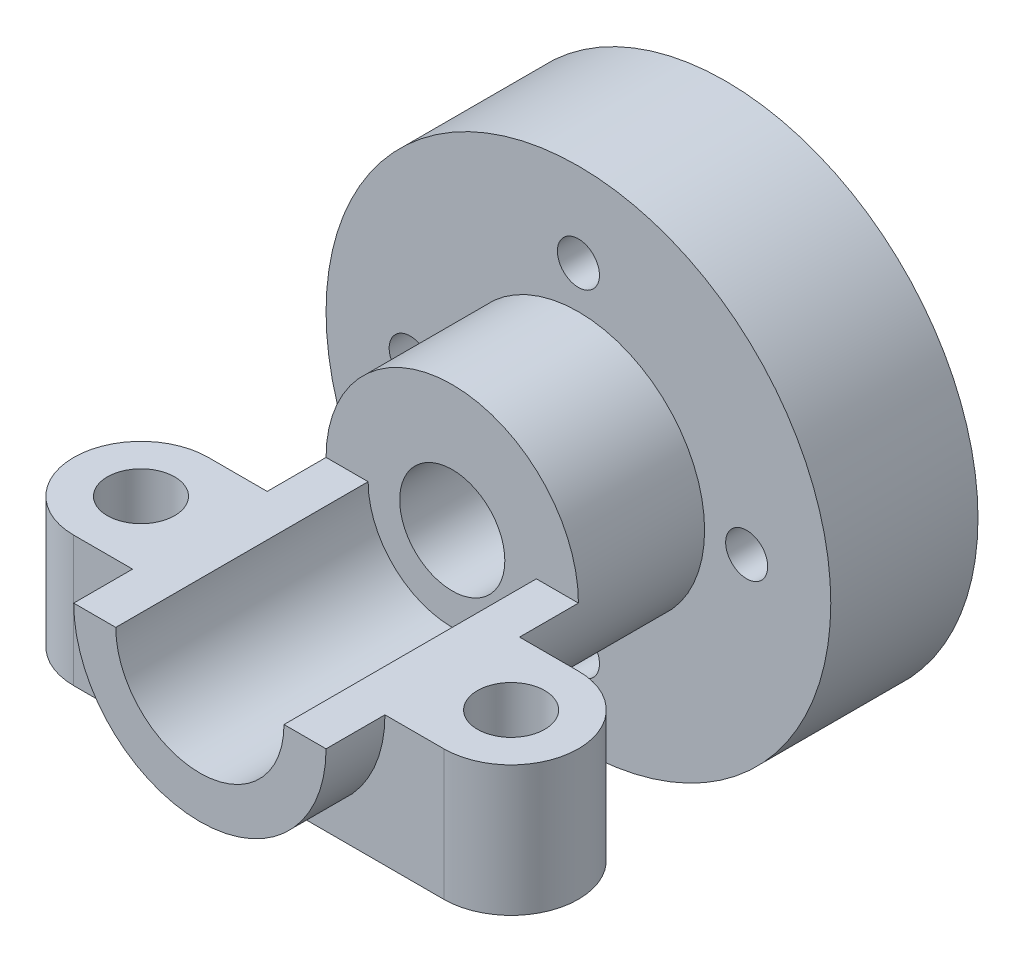
ISO-10303-21;
HEADER;
FILE_DESCRIPTION(('STEP AP214'),'2;1');
FILE_NAME('part.step','',(''),(''),'','','');
FILE_SCHEMA(('AUTOMOTIVE_DESIGN { 1 0 10303 214 1 1 1 1 }'));
ENDSEC;
DATA;
#1=APPLICATION_CONTEXT('core data for automotive mechanical design processes');
#2=APPLICATION_PROTOCOL_DEFINITION('international standard','automotive_design',2000,#1);
#3=PRODUCT_CONTEXT('',#1,'mechanical');
#4=PRODUCT('Part','Part','',(#3));
#5=PRODUCT_RELATED_PRODUCT_CATEGORY('part','',(#4));
#6=PRODUCT_DEFINITION_FORMATION('','',#4);
#7=PRODUCT_DEFINITION_CONTEXT('part definition',#1,'design');
#8=PRODUCT_DEFINITION('design','',#6,#7);
#9=PRODUCT_DEFINITION_SHAPE('','',#8);
#10=(LENGTH_UNIT() NAMED_UNIT(*) SI_UNIT(.MILLI.,.METRE.));
#11=(NAMED_UNIT(*) PLANE_ANGLE_UNIT() SI_UNIT($,.RADIAN.));
#12=(NAMED_UNIT(*) SI_UNIT($,.STERADIAN.) SOLID_ANGLE_UNIT());
#13=UNCERTAINTY_MEASURE_WITH_UNIT(LENGTH_MEASURE(1.E-05),#10,'distance_accuracy_value','');
#14=(GEOMETRIC_REPRESENTATION_CONTEXT(3) GLOBAL_UNCERTAINTY_ASSIGNED_CONTEXT((#13)) GLOBAL_UNIT_ASSIGNED_CONTEXT((#10,
#11,#12)) REPRESENTATION_CONTEXT('',''));
#15=CARTESIAN_POINT('',(0.,0.,0.));
#16=DIRECTION('',(0.,0.,1.));
#17=DIRECTION('',(1.,0.,0.));
#18=AXIS2_PLACEMENT_3D('',#15,#16,#17);
#19=CARTESIAN_POINT('',(-30.,0.,125.));
#20=DIRECTION('',(0.,-1.,0.));
#21=DIRECTION('',(0.,0.,-1.));
#22=AXIS2_PLACEMENT_3D('',#19,#20,#21);
#23=PLANE('',#22);
#24=CARTESIAN_POINT('',(44.,-1.39645239816133E-13,95.));
#25=DIRECTION('',(0.,-1.,0.));
#26=DIRECTION('',(0.,0.,-1.));
#27=AXIS2_PLACEMENT_3D('',#24,#25,#26);
#28=CIRCLE('',#27,8.);
#29=CARTESIAN_POINT('',(44.,-1.39645239816133E-13,87.));
#30=VERTEX_POINT('',#29);
#31=EDGE_CURVE('E51',#30,#30,#28,.T.);
#32=ORIENTED_EDGE('',*,*,#31,.T.);
#33=EDGE_LOOP('',(#32));
#34=FACE_BOUND('',#33,.T.);
#35=DIRECTION('',(0.,0.,1.));
#36=VECTOR('',#35,1.);
#37=CARTESIAN_POINT('',(20.,0.,65.));
#38=LINE('',#37,#36);
#39=CARTESIAN_POINT('',(20.,0.,65.));
#40=VERTEX_POINT('',#39);
#41=CARTESIAN_POINT('',(20.,0.,125.));
#42=VERTEX_POINT('',#41);
#43=EDGE_CURVE('E171',#40,#42,#38,.T.);
#44=ORIENTED_EDGE('',*,*,#43,.T.);
#45=DIRECTION('',(-1.,0.,0.));
#46=VECTOR('',#45,1.);
#47=CARTESIAN_POINT('',(12.5,0.,125.));
#48=LINE('',#47,#46);
#49=CARTESIAN_POINT('',(30.,0.,125.));
#50=VERTEX_POINT('',#49);
#51=EDGE_CURVE('E185',#50,#42,#48,.T.);
#52=ORIENTED_EDGE('',*,*,#51,.F.);
#53=DIRECTION('',(0.,0.,-1.));
#54=VECTOR('',#53,1.);
#55=CARTESIAN_POINT('',(30.,0.,125.));
#56=LINE('',#55,#54);
#57=CARTESIAN_POINT('',(30.,-1.39645239816133E-13,111.));
#58=VERTEX_POINT('',#57);
#59=EDGE_CURVE('E186',#50,#58,#56,.T.);
#60=ORIENTED_EDGE('',*,*,#59,.T.);
#61=DIRECTION('',(1.,0.,0.));
#62=VECTOR('',#61,1.);
#63=CARTESIAN_POINT('',(-60.,-1.39645239816133E-13,111.));
#64=LINE('',#63,#62);
#65=CARTESIAN_POINT('',(44.,-1.39645239816133E-13,111.));
#66=VERTEX_POINT('',#65);
#67=EDGE_CURVE('E149',#58,#66,#64,.T.);
#68=ORIENTED_EDGE('',*,*,#67,.T.);
#69=CARTESIAN_POINT('',(44.,-1.39645239816133E-13,95.));
#70=DIRECTION('',(0.,-1.,0.));
#71=DIRECTION('',(0.,0.,-1.));
#72=AXIS2_PLACEMENT_3D('',#69,#70,#71);
#73=CIRCLE('',#72,16.);
#74=CARTESIAN_POINT('',(44.,-1.39645239816133E-13,79.));
#75=VERTEX_POINT('',#74);
#76=EDGE_CURVE('E137',#66,#75,#73,.F.);
#77=ORIENTED_EDGE('',*,*,#76,.T.);
#78=DIRECTION('',(1.,0.,0.));
#79=VECTOR('',#78,1.);
#80=CARTESIAN_POINT('',(-60.,-1.39645239816133E-13,79.));
#81=LINE('',#80,#79);
#82=CARTESIAN_POINT('',(30.,-1.39645239816133E-13,79.));
#83=VERTEX_POINT('',#82);
#84=EDGE_CURVE('E146',#83,#75,#81,.T.);
#85=ORIENTED_EDGE('',*,*,#84,.F.);
#86=CARTESIAN_POINT('',(30.,0.,65.));
#87=VERTEX_POINT('',#86);
#88=EDGE_CURVE('E66',#83,#87,#56,.T.);
#89=ORIENTED_EDGE('',*,*,#88,.T.);
#90=DIRECTION('',(-1.,0.,0.));
#91=VECTOR('',#90,1.);
#92=CARTESIAN_POINT('',(12.5,0.,65.));
#93=LINE('',#92,#91);
#94=EDGE_CURVE('E176',#87,#40,#93,.T.);
#95=ORIENTED_EDGE('',*,*,#94,.T.);
#96=EDGE_LOOP('',(#44,#52,#60,#68,#77,#85,#89,#95));
#97=FACE_BOUND('',#96,.T.);
#98=ADVANCED_FACE('F50',(#34,#97),#23,.F.);
#99=CARTESIAN_POINT('',(0.,1.,111.));
#100=DIRECTION('',(0.,0.,1.));
#101=DIRECTION('',(1.,0.,0.));
#102=AXIS2_PLACEMENT_3D('',#99,#100,#101);
#103=PLANE('',#102);
#104=CARTESIAN_POINT('',(-44.,-1.39645239816133E-13,111.));
#105=VERTEX_POINT('',#104);
#106=CARTESIAN_POINT('',(-30.,0.,111.));
#107=VERTEX_POINT('',#106);
#108=EDGE_CURVE('E128',#105,#107,#64,.T.);
#109=ORIENTED_EDGE('',*,*,#108,.F.);
#110=DIRECTION('',(0.,-1.,0.));
#111=VECTOR('',#110,1.);
#112=CARTESIAN_POINT('',(-44.,1.,111.));
#113=LINE('',#112,#111);
#114=CARTESIAN_POINT('',(-44.,-31.,111.));
#115=VERTEX_POINT('',#114);
#116=EDGE_CURVE('E141',#105,#115,#113,.T.);
#117=ORIENTED_EDGE('',*,*,#116,.T.);
#118=DIRECTION('',(-1.,0.,0.));
#119=VECTOR('',#118,1.);
#120=CARTESIAN_POINT('',(0.,-31.,111.));
#121=LINE('',#120,#119);
#122=CARTESIAN_POINT('',(44.,-31.,111.));
#123=VERTEX_POINT('',#122);
#124=EDGE_CURVE('E328',#123,#115,#121,.T.);
#125=ORIENTED_EDGE('',*,*,#124,.F.);
#126=DIRECTION('',(0.,-1.,0.));
#127=VECTOR('',#126,1.);
#128=CARTESIAN_POINT('',(44.,1.,111.));
#129=LINE('',#128,#127);
#130=EDGE_CURVE('E156',#66,#123,#129,.T.);
#131=ORIENTED_EDGE('',*,*,#130,.F.);
#132=ORIENTED_EDGE('',*,*,#67,.F.);
#133=CARTESIAN_POINT('',(0.,0.,111.));
#134=DIRECTION('',(0.,0.,1.));
#135=DIRECTION('',(1.,0.,0.));
#136=AXIS2_PLACEMENT_3D('',#133,#134,#135);
#137=CIRCLE('',#136,30.);
#138=EDGE_CURVE('E148',#107,#58,#137,.T.);
#139=ORIENTED_EDGE('',*,*,#138,.F.);
#140=EDGE_LOOP('',(#109,#117,#125,#131,#132,#139));
#141=FACE_BOUND('',#140,.T.);
#142=ADVANCED_FACE('F143',(#141),#103,.T.);
#143=CARTESIAN_POINT('',(0.,1.,79.));
#144=DIRECTION('',(0.,0.,-1.));
#145=DIRECTION('',(-1.,0.,0.));
#146=AXIS2_PLACEMENT_3D('',#143,#144,#145);
#147=PLANE('',#146);
#148=ORIENTED_EDGE('',*,*,#84,.T.);
#149=DIRECTION('',(0.,-1.,0.));
#150=VECTOR('',#149,1.);
#151=CARTESIAN_POINT('',(44.,1.,79.));
#152=LINE('',#151,#150);
#153=CARTESIAN_POINT('',(44.,-31.,79.));
#154=VERTEX_POINT('',#153);
#155=EDGE_CURVE('E159',#75,#154,#152,.T.);
#156=ORIENTED_EDGE('',*,*,#155,.T.);
#157=DIRECTION('',(1.,0.,0.));
#158=VECTOR('',#157,1.);
#159=CARTESIAN_POINT('',(0.,-31.,79.));
#160=LINE('',#159,#158);
#161=CARTESIAN_POINT('',(-44.,-31.,79.));
#162=VERTEX_POINT('',#161);
#163=EDGE_CURVE('E322',#162,#154,#160,.T.);
#164=ORIENTED_EDGE('',*,*,#163,.F.);
#165=DIRECTION('',(0.,-1.,0.));
#166=VECTOR('',#165,1.);
#167=CARTESIAN_POINT('',(-44.,1.,79.));
#168=LINE('',#167,#166);
#169=CARTESIAN_POINT('',(-44.,-1.39645239816133E-13,79.));
#170=VERTEX_POINT('',#169);
#171=EDGE_CURVE('E170',#170,#162,#168,.T.);
#172=ORIENTED_EDGE('',*,*,#171,.F.);
#173=CARTESIAN_POINT('',(-30.,-1.39645239816133E-13,79.));
#174=VERTEX_POINT('',#173);
#175=EDGE_CURVE('E131',#170,#174,#81,.T.);
#176=ORIENTED_EDGE('',*,*,#175,.T.);
#177=CARTESIAN_POINT('',(0.,0.,79.));
#178=DIRECTION('',(0.,0.,-1.));
#179=DIRECTION('',(-1.,0.,0.));
#180=AXIS2_PLACEMENT_3D('',#177,#178,#179);
#181=CIRCLE('',#180,30.);
#182=EDGE_CURVE('E154',#83,#174,#181,.T.);
#183=ORIENTED_EDGE('',*,*,#182,.F.);
#184=EDGE_LOOP('',(#148,#156,#164,#172,#176,#183));
#185=FACE_BOUND('',#184,.T.);
#186=ADVANCED_FACE('F250',(#185),#147,.T.);
#187=CARTESIAN_POINT('',(0.,0.,65.));
#188=DIRECTION('',(0.,0.,-1.));
#189=DIRECTION('',(-1.,0.,0.));
#190=AXIS2_PLACEMENT_3D('',#187,#188,#189);
#191=CYLINDRICAL_SURFACE('',#190,12.5);
#192=CARTESIAN_POINT('',(0.,0.,15.));
#193=DIRECTION('',(0.,0.,1.));
#194=DIRECTION('',(1.,0.,0.));
#195=AXIS2_PLACEMENT_3D('',#192,#193,#194);
#196=CIRCLE('',#195,12.5);
#197=CARTESIAN_POINT('',(12.5,0.,15.));
#198=VERTEX_POINT('',#197);
#199=EDGE_CURVE('E195',#198,#198,#196,.T.);
#200=ORIENTED_EDGE('',*,*,#199,.F.);
#201=EDGE_LOOP('',(#200));
#202=FACE_BOUND('',#201,.T.);
#203=CARTESIAN_POINT('',(0.,0.,65.));
#204=DIRECTION('',(0.,0.,1.));
#205=DIRECTION('',(1.,0.,0.));
#206=AXIS2_PLACEMENT_3D('',#203,#204,#205);
#207=CIRCLE('',#206,12.5);
#208=CARTESIAN_POINT('',(12.5,0.,65.));
#209=VERTEX_POINT('',#208);
#210=EDGE_CURVE('E191',#209,#209,#207,.T.);
#211=ORIENTED_EDGE('',*,*,#210,.T.);
#212=EDGE_LOOP('',(#211));
#213=FACE_BOUND('',#212,.T.);
#214=ADVANCED_FACE('F244',(#202,#213),#191,.F.);
#215=CARTESIAN_POINT('',(0.,0.,0.));
#216=DIRECTION('',(0.,0.,1.));
#217=DIRECTION('',(1.,0.,0.));
#218=AXIS2_PLACEMENT_3D('',#215,#216,#217);
#219=PLANE('',#218);
#220=CARTESIAN_POINT('',(0.,0.,0.));
#221=DIRECTION('',(0.,0.,1.));
#222=DIRECTION('',(1.,0.,0.));
#223=AXIS2_PLACEMENT_3D('',#220,#221,#222);
#224=CIRCLE('',#223,60.);
#225=CARTESIAN_POINT('',(60.,0.,0.));
#226=VERTEX_POINT('',#225);
#227=EDGE_CURVE('E57',#226,#226,#224,.T.);
#228=ORIENTED_EDGE('',*,*,#227,.F.);
#229=EDGE_LOOP('',(#228));
#230=FACE_BOUND('',#229,.T.);
#231=CARTESIAN_POINT('',(0.,0.,0.));
#232=DIRECTION('',(0.,0.,1.));
#233=DIRECTION('',(1.,0.,0.));
#234=AXIS2_PLACEMENT_3D('',#231,#232,#233);
#235=CIRCLE('',#234,55.);
#236=CARTESIAN_POINT('',(55.,0.,0.));
#237=VERTEX_POINT('',#236);
#238=EDGE_CURVE('E235',#237,#237,#235,.T.);
#239=ORIENTED_EDGE('',*,*,#238,.T.);
#240=EDGE_LOOP('',(#239));
#241=FACE_BOUND('',#240,.T.);
#242=ADVANCED_FACE('F247',(#230,#241),#219,.F.);
#243=CARTESIAN_POINT('',(0.,0.,15.));
#244=DIRECTION('',(0.,0.,-1.));
#245=DIRECTION('',(-1.,0.,0.));
#246=AXIS2_PLACEMENT_3D('',#243,#244,#245);
#247=CYLINDRICAL_SURFACE('',#246,60.);
#248=ORIENTED_EDGE('',*,*,#227,.T.);
#249=EDGE_LOOP('',(#248));
#250=FACE_BOUND('',#249,.T.);
#251=CARTESIAN_POINT('',(0.,0.,35.));
#252=DIRECTION('',(0.,0.,1.));
#253=DIRECTION('',(1.,0.,0.));
#254=AXIS2_PLACEMENT_3D('',#251,#252,#253);
#255=CIRCLE('',#254,60.);
#256=CARTESIAN_POINT('',(60.,0.,35.));
#257=VERTEX_POINT('',#256);
#258=EDGE_CURVE('E208',#257,#257,#255,.T.);
#259=ORIENTED_EDGE('',*,*,#258,.F.);
#260=EDGE_LOOP('',(#259));
#261=FACE_BOUND('',#260,.T.);
#262=ADVANCED_FACE('F47',(#250,#261),#247,.T.);
#263=CARTESIAN_POINT('',(0.,0.,15.));
#264=DIRECTION('',(0.,0.,-1.));
#265=DIRECTION('',(-1.,0.,0.));
#266=AXIS2_PLACEMENT_3D('',#263,#264,#265);
#267=CYLINDRICAL_SURFACE('',#266,55.);
#268=CARTESIAN_POINT('',(0.,0.,15.));
#269=DIRECTION('',(0.,0.,1.));
#270=DIRECTION('',(1.,0.,0.));
#271=AXIS2_PLACEMENT_3D('',#268,#269,#270);
#272=CIRCLE('',#271,55.);
#273=CARTESIAN_POINT('',(55.,0.,15.));
#274=VERTEX_POINT('',#273);
#275=EDGE_CURVE('E233',#274,#274,#272,.T.);
#276=ORIENTED_EDGE('',*,*,#275,.T.);
#277=EDGE_LOOP('',(#276));
#278=FACE_BOUND('',#277,.T.);
#279=ORIENTED_EDGE('',*,*,#238,.F.);
#280=EDGE_LOOP('',(#279));
#281=FACE_BOUND('',#280,.T.);
#282=ADVANCED_FACE('F356',(#278,#281),#267,.F.);
#283=CARTESIAN_POINT('',(0.,0.,15.));
#284=DIRECTION('',(0.,0.,1.));
#285=DIRECTION('',(1.,0.,0.));
#286=AXIS2_PLACEMENT_3D('',#283,#284,#285);
#287=PLANE('',#286);
#288=ORIENTED_EDGE('',*,*,#199,.T.);
#289=EDGE_LOOP('',(#288));
#290=FACE_BOUND('',#289,.T.);
#291=CARTESIAN_POINT('',(0.,40.,15.));
#292=DIRECTION('',(0.,0.,1.));
#293=DIRECTION('',(1.,0.,0.));
#294=AXIS2_PLACEMENT_3D('',#291,#292,#293);
#295=CIRCLE('',#294,5.);
#296=CARTESIAN_POINT('',(5.,40.,15.));
#297=VERTEX_POINT('',#296);
#298=EDGE_CURVE('E202',#297,#297,#295,.T.);
#299=ORIENTED_EDGE('',*,*,#298,.T.);
#300=EDGE_LOOP('',(#299));
#301=FACE_BOUND('',#300,.T.);
#302=CARTESIAN_POINT('',(40.0000000000011,1.12952049642128E-12,15.));
#303=DIRECTION('',(0.,0.,1.));
#304=DIRECTION('',(1.,0.,0.));
#305=AXIS2_PLACEMENT_3D('',#302,#303,#304);
#306=CIRCLE('',#305,5.);
#307=CARTESIAN_POINT('',(45.0000000000011,1.12952049642128E-12,15.));
#308=VERTEX_POINT('',#307);
#309=EDGE_CURVE('E215',#308,#308,#306,.T.);
#310=ORIENTED_EDGE('',*,*,#309,.T.);
#311=EDGE_LOOP('',(#310));
#312=FACE_BOUND('',#311,.T.);
#313=CARTESIAN_POINT('',(2.25904099284255E-12,-40.,15.));
#314=DIRECTION('',(0.,0.,1.));
#315=DIRECTION('',(1.,0.,0.));
#316=AXIS2_PLACEMENT_3D('',#313,#314,#315);
#317=CIRCLE('',#316,5.);
#318=CARTESIAN_POINT('',(5.00000000000226,-40.,15.));
#319=VERTEX_POINT('',#318);
#320=EDGE_CURVE('E217',#319,#319,#317,.T.);
#321=ORIENTED_EDGE('',*,*,#320,.T.);
#322=EDGE_LOOP('',(#321));
#323=FACE_BOUND('',#322,.T.);
#324=CARTESIAN_POINT('',(-39.9999999999989,-1.13441908361787E-12,15.));
#325=DIRECTION('',(0.,0.,1.));
#326=DIRECTION('',(1.,0.,0.));
#327=AXIS2_PLACEMENT_3D('',#324,#325,#326);
#328=CIRCLE('',#327,5.);
#329=CARTESIAN_POINT('',(-34.9999999999989,-1.13441908361787E-12,15.));
#330=VERTEX_POINT('',#329);
#331=EDGE_CURVE('E221',#330,#330,#328,.T.);
#332=ORIENTED_EDGE('',*,*,#331,.T.);
#333=EDGE_LOOP('',(#332));
#334=FACE_BOUND('',#333,.T.);
#335=ORIENTED_EDGE('',*,*,#275,.F.);
#336=EDGE_LOOP('',(#335));
#337=FACE_BOUND('',#336,.T.);
#338=ADVANCED_FACE('F245',(#290,#301,#312,#323,#334,#337),#287,.F.);
#339=CARTESIAN_POINT('',(0.,0.,35.));
#340=DIRECTION('',(0.,0.,1.));
#341=DIRECTION('',(1.,0.,0.));
#342=AXIS2_PLACEMENT_3D('',#339,#340,#341);
#343=PLANE('',#342);
#344=CARTESIAN_POINT('',(0.,0.,35.));
#345=DIRECTION('',(0.,0.,1.));
#346=DIRECTION('',(1.,0.,0.));
#347=AXIS2_PLACEMENT_3D('',#344,#345,#346);
#348=CIRCLE('',#347,30.);
#349=CARTESIAN_POINT('',(30.,0.,35.));
#350=VERTEX_POINT('',#349);
#351=EDGE_CURVE('E196',#350,#350,#348,.T.);
#352=ORIENTED_EDGE('',*,*,#351,.F.);
#353=EDGE_LOOP('',(#352));
#354=FACE_BOUND('',#353,.T.);
#355=CARTESIAN_POINT('',(0.,40.,35.));
#356=DIRECTION('',(0.,0.,1.));
#357=DIRECTION('',(1.,0.,0.));
#358=AXIS2_PLACEMENT_3D('',#355,#356,#357);
#359=CIRCLE('',#358,5.);
#360=CARTESIAN_POINT('',(5.,40.,35.));
#361=VERTEX_POINT('',#360);
#362=EDGE_CURVE('E207',#361,#361,#359,.T.);
#363=ORIENTED_EDGE('',*,*,#362,.F.);
#364=EDGE_LOOP('',(#363));
#365=FACE_BOUND('',#364,.T.);
#366=CARTESIAN_POINT('',(40.0000000000011,1.12952049642128E-12,35.));
#367=DIRECTION('',(0.,0.,1.));
#368=DIRECTION('',(1.,0.,0.));
#369=AXIS2_PLACEMENT_3D('',#366,#367,#368);
#370=CIRCLE('',#369,5.);
#371=CARTESIAN_POINT('',(45.0000000000011,1.12952049642128E-12,35.));
#372=VERTEX_POINT('',#371);
#373=EDGE_CURVE('E214',#372,#372,#370,.T.);
#374=ORIENTED_EDGE('',*,*,#373,.F.);
#375=EDGE_LOOP('',(#374));
#376=FACE_BOUND('',#375,.T.);
#377=CARTESIAN_POINT('',(2.25904099284255E-12,-40.,35.));
#378=DIRECTION('',(0.,0.,1.));
#379=DIRECTION('',(1.,0.,0.));
#380=AXIS2_PLACEMENT_3D('',#377,#378,#379);
#381=CIRCLE('',#380,5.);
#382=CARTESIAN_POINT('',(5.00000000000226,-40.,35.));
#383=VERTEX_POINT('',#382);
#384=EDGE_CURVE('E222',#383,#383,#381,.T.);
#385=ORIENTED_EDGE('',*,*,#384,.F.);
#386=EDGE_LOOP('',(#385));
#387=FACE_BOUND('',#386,.T.);
#388=CARTESIAN_POINT('',(-39.9999999999989,-1.13441908361787E-12,35.));
#389=DIRECTION('',(0.,0.,1.));
#390=DIRECTION('',(1.,0.,0.));
#391=AXIS2_PLACEMENT_3D('',#388,#389,#390);
#392=CIRCLE('',#391,5.);
#393=CARTESIAN_POINT('',(-34.9999999999989,-1.13441908361787E-12,35.));
#394=VERTEX_POINT('',#393);
#395=EDGE_CURVE('E205',#394,#394,#392,.T.);
#396=ORIENTED_EDGE('',*,*,#395,.F.);
#397=EDGE_LOOP('',(#396));
#398=FACE_BOUND('',#397,.T.);
#399=ORIENTED_EDGE('',*,*,#258,.T.);
#400=EDGE_LOOP('',(#399));
#401=FACE_BOUND('',#400,.T.);
#402=ADVANCED_FACE('F367',(#354,#365,#376,#387,#398,#401),#343,.T.);
#403=CARTESIAN_POINT('',(-39.9999999999989,-1.13441908361787E-12,15.));
#404=DIRECTION('',(0.,0.,1.));
#405=DIRECTION('',(1.,0.,0.));
#406=AXIS2_PLACEMENT_3D('',#403,#404,#405);
#407=CYLINDRICAL_SURFACE('',#406,5.);
#408=ORIENTED_EDGE('',*,*,#331,.F.);
#409=EDGE_LOOP('',(#408));
#410=FACE_BOUND('',#409,.T.);
#411=ORIENTED_EDGE('',*,*,#395,.T.);
#412=EDGE_LOOP('',(#411));
#413=FACE_BOUND('',#412,.T.);
#414=ADVANCED_FACE('F374',(#410,#413),#407,.F.);
#415=CARTESIAN_POINT('',(2.25904099284255E-12,-40.,15.));
#416=DIRECTION('',(0.,0.,1.));
#417=DIRECTION('',(1.,0.,0.));
#418=AXIS2_PLACEMENT_3D('',#415,#416,#417);
#419=CYLINDRICAL_SURFACE('',#418,5.);
#420=ORIENTED_EDGE('',*,*,#320,.F.);
#421=EDGE_LOOP('',(#420));
#422=FACE_BOUND('',#421,.T.);
#423=ORIENTED_EDGE('',*,*,#384,.T.);
#424=EDGE_LOOP('',(#423));
#425=FACE_BOUND('',#424,.T.);
#426=ADVANCED_FACE('F378',(#422,#425),#419,.F.);
#427=CARTESIAN_POINT('',(40.0000000000011,1.12952049642128E-12,15.));
#428=DIRECTION('',(0.,0.,1.));
#429=DIRECTION('',(1.,0.,0.));
#430=AXIS2_PLACEMENT_3D('',#427,#428,#429);
#431=CYLINDRICAL_SURFACE('',#430,5.);
#432=ORIENTED_EDGE('',*,*,#309,.F.);
#433=EDGE_LOOP('',(#432));
#434=FACE_BOUND('',#433,.T.);
#435=ORIENTED_EDGE('',*,*,#373,.T.);
#436=EDGE_LOOP('',(#435));
#437=FACE_BOUND('',#436,.T.);
#438=ADVANCED_FACE('F266',(#434,#437),#431,.F.);
#439=CARTESIAN_POINT('',(0.,40.,15.));
#440=DIRECTION('',(0.,0.,1.));
#441=DIRECTION('',(1.,0.,0.));
#442=AXIS2_PLACEMENT_3D('',#439,#440,#441);
#443=CYLINDRICAL_SURFACE('',#442,5.);
#444=ORIENTED_EDGE('',*,*,#298,.F.);
#445=EDGE_LOOP('',(#444));
#446=FACE_BOUND('',#445,.T.);
#447=ORIENTED_EDGE('',*,*,#362,.T.);
#448=EDGE_LOOP('',(#447));
#449=FACE_BOUND('',#448,.T.);
#450=ADVANCED_FACE('F258',(#446,#449),#443,.F.);
#451=CARTESIAN_POINT('',(0.,0.,65.));
#452=DIRECTION('',(0.,0.,1.));
#453=DIRECTION('',(1.,0.,0.));
#454=AXIS2_PLACEMENT_3D('',#451,#452,#453);
#455=PLANE('',#454);
#456=DIRECTION('',(-1.,0.,0.));
#457=VECTOR('',#456,1.);
#458=CARTESIAN_POINT('',(-30.,0.,65.));
#459=LINE('',#458,#457);
#460=CARTESIAN_POINT('',(-20.,0.,65.));
#461=VERTEX_POINT('',#460);
#462=CARTESIAN_POINT('',(-30.,0.,65.));
#463=VERTEX_POINT('',#462);
#464=EDGE_CURVE('E178',#461,#463,#459,.T.);
#465=ORIENTED_EDGE('',*,*,#464,.F.);
#466=CARTESIAN_POINT('',(0.,0.,65.));
#467=DIRECTION('',(0.,0.,1.));
#468=DIRECTION('',(1.,0.,0.));
#469=AXIS2_PLACEMENT_3D('',#466,#467,#468);
#470=CIRCLE('',#469,20.);
#471=EDGE_CURVE('E168',#461,#40,#470,.T.);
#472=ORIENTED_EDGE('',*,*,#471,.T.);
#473=ORIENTED_EDGE('',*,*,#94,.F.);
#474=CARTESIAN_POINT('',(0.,0.,65.));
#475=DIRECTION('',(0.,0.,1.));
#476=DIRECTION('',(1.,0.,0.));
#477=AXIS2_PLACEMENT_3D('',#474,#475,#476);
#478=CIRCLE('',#477,30.);
#479=EDGE_CURVE('E200',#87,#463,#478,.T.);
#480=ORIENTED_EDGE('',*,*,#479,.T.);
#481=EDGE_LOOP('',(#465,#472,#473,#480));
#482=FACE_BOUND('',#481,.T.);
#483=ORIENTED_EDGE('',*,*,#210,.F.);
#484=EDGE_LOOP('',(#483));
#485=FACE_BOUND('',#484,.T.);
#486=ADVANCED_FACE('F251',(#482,#485),#455,.T.);
#487=CARTESIAN_POINT('',(0.,0.,65.));
#488=DIRECTION('',(0.,0.,-1.));
#489=DIRECTION('',(-1.,0.,0.));
#490=AXIS2_PLACEMENT_3D('',#487,#488,#489);
#491=CYLINDRICAL_SURFACE('',#490,30.);
#492=ORIENTED_EDGE('',*,*,#88,.F.);
#493=ORIENTED_EDGE('',*,*,#182,.T.);
#494=DIRECTION('',(0.,0.,-1.));
#495=VECTOR('',#494,1.);
#496=CARTESIAN_POINT('',(-30.,0.,125.));
#497=LINE('',#496,#495);
#498=EDGE_CURVE('E193',#174,#463,#497,.T.);
#499=ORIENTED_EDGE('',*,*,#498,.T.);
#500=ORIENTED_EDGE('',*,*,#479,.F.);
#501=EDGE_LOOP('',(#492,#493,#499,#500));
#502=FACE_BOUND('',#501,.T.);
#503=ORIENTED_EDGE('',*,*,#351,.T.);
#504=EDGE_LOOP('',(#503));
#505=FACE_BOUND('',#504,.T.);
#506=ADVANCED_FACE('F254',(#502,#505),#491,.T.);
#507=DIRECTION('',(0.,0.,1.));
#508=VECTOR('',#507,1.);
#509=CARTESIAN_POINT('',(-20.,0.,65.));
#510=LINE('',#509,#508);
#511=CARTESIAN_POINT('',(-20.,0.,125.));
#512=VERTEX_POINT('',#511);
#513=EDGE_CURVE('E65',#512,#461,#510,.F.);
#514=ORIENTED_EDGE('',*,*,#513,.T.);
#515=ORIENTED_EDGE('',*,*,#464,.T.);
#516=ORIENTED_EDGE('',*,*,#498,.F.);
#517=ORIENTED_EDGE('',*,*,#175,.F.);
#518=CARTESIAN_POINT('',(-44.,-1.39645239816133E-13,95.));
#519=DIRECTION('',(0.,-1.,0.));
#520=DIRECTION('',(0.,0.,-1.));
#521=AXIS2_PLACEMENT_3D('',#518,#519,#520);
#522=CIRCLE('',#521,16.);
#523=EDGE_CURVE('E121',#170,#105,#522,.F.);
#524=ORIENTED_EDGE('',*,*,#523,.T.);
#525=ORIENTED_EDGE('',*,*,#108,.T.);
#526=CARTESIAN_POINT('',(-30.,0.,125.));
#527=VERTEX_POINT('',#526);
#528=EDGE_CURVE('E194',#527,#107,#497,.T.);
#529=ORIENTED_EDGE('',*,*,#528,.F.);
#530=DIRECTION('',(-1.,0.,0.));
#531=VECTOR('',#530,1.);
#532=CARTESIAN_POINT('',(-30.,0.,125.));
#533=LINE('',#532,#531);
#534=EDGE_CURVE('E179',#512,#527,#533,.T.);
#535=ORIENTED_EDGE('',*,*,#534,.F.);
#536=EDGE_LOOP('',(#514,#515,#516,#517,#524,#525,#529,#535));
#537=FACE_BOUND('',#536,.T.);
#538=CARTESIAN_POINT('',(-44.,-1.39645239816133E-13,95.));
#539=DIRECTION('',(0.,-1.,0.));
#540=DIRECTION('',(0.,0.,-1.));
#541=AXIS2_PLACEMENT_3D('',#538,#539,#540);
#542=CIRCLE('',#541,8.);
#543=CARTESIAN_POINT('',(-44.,-1.39645239816133E-13,87.));
#544=VERTEX_POINT('',#543);
#545=EDGE_CURVE('E316',#544,#544,#542,.T.);
#546=ORIENTED_EDGE('',*,*,#545,.T.);
#547=EDGE_LOOP('',(#546));
#548=FACE_BOUND('',#547,.T.);
#549=ADVANCED_FACE('F130',(#537,#548),#23,.F.);
#550=CARTESIAN_POINT('',(0.,0.,65.));
#551=DIRECTION('',(0.,0.,1.));
#552=DIRECTION('',(1.,0.,0.));
#553=AXIS2_PLACEMENT_3D('',#550,#551,#552);
#554=CYLINDRICAL_SURFACE('',#553,20.);
#555=ORIENTED_EDGE('',*,*,#471,.F.);
#556=ORIENTED_EDGE('',*,*,#513,.F.);
#557=CARTESIAN_POINT('',(0.,0.,125.));
#558=DIRECTION('',(0.,0.,1.));
#559=DIRECTION('',(1.,0.,0.));
#560=AXIS2_PLACEMENT_3D('',#557,#558,#559);
#561=CIRCLE('',#560,20.);
#562=EDGE_CURVE('E11',#512,#42,#561,.T.);
#563=ORIENTED_EDGE('',*,*,#562,.T.);
#564=ORIENTED_EDGE('',*,*,#43,.F.);
#565=EDGE_LOOP('',(#555,#556,#563,#564));
#566=FACE_BOUND('',#565,.T.);
#567=ADVANCED_FACE('F278',(#566),#554,.F.);
#568=CARTESIAN_POINT('',(-44.,1.,95.));
#569=DIRECTION('',(0.,-1.,0.));
#570=DIRECTION('',(0.,0.,-1.));
#571=AXIS2_PLACEMENT_3D('',#568,#569,#570);
#572=CYLINDRICAL_SURFACE('',#571,16.);
#573=ORIENTED_EDGE('',*,*,#523,.F.);
#574=ORIENTED_EDGE('',*,*,#171,.T.);
#575=CARTESIAN_POINT('',(-44.,-31.,95.));
#576=DIRECTION('',(0.,-1.,0.));
#577=DIRECTION('',(0.,0.,-1.));
#578=AXIS2_PLACEMENT_3D('',#575,#576,#577);
#579=CIRCLE('',#578,16.);
#580=EDGE_CURVE('E153',#115,#162,#579,.T.);
#581=ORIENTED_EDGE('',*,*,#580,.F.);
#582=ORIENTED_EDGE('',*,*,#116,.F.);
#583=EDGE_LOOP('',(#573,#574,#581,#582));
#584=FACE_BOUND('',#583,.T.);
#585=ADVANCED_FACE('F151',(#584),#572,.T.);
#586=CARTESIAN_POINT('',(44.,1.,95.));
#587=DIRECTION('',(0.,-1.,0.));
#588=DIRECTION('',(0.,0.,-1.));
#589=AXIS2_PLACEMENT_3D('',#586,#587,#588);
#590=CYLINDRICAL_SURFACE('',#589,16.);
#591=ORIENTED_EDGE('',*,*,#76,.F.);
#592=ORIENTED_EDGE('',*,*,#130,.T.);
#593=CARTESIAN_POINT('',(44.,-31.,95.));
#594=DIRECTION('',(0.,-1.,0.));
#595=DIRECTION('',(0.,0.,-1.));
#596=AXIS2_PLACEMENT_3D('',#593,#594,#595);
#597=CIRCLE('',#596,16.);
#598=EDGE_CURVE('E330',#154,#123,#597,.T.);
#599=ORIENTED_EDGE('',*,*,#598,.F.);
#600=ORIENTED_EDGE('',*,*,#155,.F.);
#601=EDGE_LOOP('',(#591,#592,#599,#600));
#602=FACE_BOUND('',#601,.T.);
#603=ADVANCED_FACE('F287',(#602),#590,.T.);
#604=CARTESIAN_POINT('',(-44.,1.,95.));
#605=DIRECTION('',(0.,-1.,0.));
#606=DIRECTION('',(0.,0.,-1.));
#607=AXIS2_PLACEMENT_3D('',#604,#605,#606);
#608=CYLINDRICAL_SURFACE('',#607,8.);
#609=ORIENTED_EDGE('',*,*,#545,.F.);
#610=EDGE_LOOP('',(#609));
#611=FACE_BOUND('',#610,.T.);
#612=CARTESIAN_POINT('',(-44.,-31.,95.));
#613=DIRECTION('',(0.,-1.,0.));
#614=DIRECTION('',(0.,0.,-1.));
#615=AXIS2_PLACEMENT_3D('',#612,#613,#614);
#616=CIRCLE('',#615,8.);
#617=CARTESIAN_POINT('',(-44.,-31.,87.));
#618=VERTEX_POINT('',#617);
#619=EDGE_CURVE('E139',#618,#618,#616,.F.);
#620=ORIENTED_EDGE('',*,*,#619,.F.);
#621=EDGE_LOOP('',(#620));
#622=FACE_BOUND('',#621,.T.);
#623=ADVANCED_FACE('F292',(#611,#622),#608,.F.);
#624=CARTESIAN_POINT('',(44.,1.,95.));
#625=DIRECTION('',(0.,-1.,0.));
#626=DIRECTION('',(0.,0.,-1.));
#627=AXIS2_PLACEMENT_3D('',#624,#625,#626);
#628=CYLINDRICAL_SURFACE('',#627,8.);
#629=ORIENTED_EDGE('',*,*,#31,.F.);
#630=EDGE_LOOP('',(#629));
#631=FACE_BOUND('',#630,.T.);
#632=CARTESIAN_POINT('',(44.,-31.,95.));
#633=DIRECTION('',(0.,-1.,0.));
#634=DIRECTION('',(0.,0.,-1.));
#635=AXIS2_PLACEMENT_3D('',#632,#633,#634);
#636=CIRCLE('',#635,8.);
#637=CARTESIAN_POINT('',(44.,-31.,87.));
#638=VERTEX_POINT('',#637);
#639=EDGE_CURVE('E162',#638,#638,#636,.F.);
#640=ORIENTED_EDGE('',*,*,#639,.F.);
#641=EDGE_LOOP('',(#640));
#642=FACE_BOUND('',#641,.T.);
#643=ADVANCED_FACE('F303',(#631,#642),#628,.F.);
#644=CARTESIAN_POINT('',(0.,-31.,0.));
#645=DIRECTION('',(0.,-1.,0.));
#646=DIRECTION('',(0.,0.,-1.));
#647=AXIS2_PLACEMENT_3D('',#644,#645,#646);
#648=PLANE('',#647);
#649=ORIENTED_EDGE('',*,*,#619,.T.);
#650=EDGE_LOOP('',(#649));
#651=FACE_BOUND('',#650,.T.);
#652=ORIENTED_EDGE('',*,*,#580,.T.);
#653=ORIENTED_EDGE('',*,*,#163,.T.);
#654=ORIENTED_EDGE('',*,*,#598,.T.);
#655=ORIENTED_EDGE('',*,*,#124,.T.);
#656=EDGE_LOOP('',(#652,#653,#654,#655));
#657=FACE_BOUND('',#656,.T.);
#658=ORIENTED_EDGE('',*,*,#639,.T.);
#659=EDGE_LOOP('',(#658));
#660=FACE_BOUND('',#659,.T.);
#661=ADVANCED_FACE('F294',(#651,#657,#660),#648,.T.);
#662=CARTESIAN_POINT('',(0.,0.,125.));
#663=DIRECTION('',(0.,0.,1.));
#664=DIRECTION('',(1.,0.,0.));
#665=AXIS2_PLACEMENT_3D('',#662,#663,#664);
#666=PLANE('',#665);
#667=ORIENTED_EDGE('',*,*,#562,.F.);
#668=ORIENTED_EDGE('',*,*,#534,.T.);
#669=CARTESIAN_POINT('',(0.,0.,125.));
#670=DIRECTION('',(0.,0.,1.));
#671=DIRECTION('',(1.,0.,0.));
#672=AXIS2_PLACEMENT_3D('',#669,#670,#671);
#673=CIRCLE('',#672,30.);
#674=EDGE_CURVE('E180',#527,#50,#673,.T.);
#675=ORIENTED_EDGE('',*,*,#674,.T.);
#676=ORIENTED_EDGE('',*,*,#51,.T.);
#677=EDGE_LOOP('',(#667,#668,#675,#676));
#678=FACE_BOUND('',#677,.T.);
#679=ADVANCED_FACE('F295',(#678),#666,.T.);
#680=ORIENTED_EDGE('',*,*,#528,.T.);
#681=ORIENTED_EDGE('',*,*,#138,.T.);
#682=ORIENTED_EDGE('',*,*,#59,.F.);
#683=ORIENTED_EDGE('',*,*,#674,.F.);
#684=EDGE_LOOP('',(#680,#681,#682,#683));
#685=FACE_BOUND('',#684,.T.);
#686=ADVANCED_FACE('F264',(#685),#491,.T.);
#687=CLOSED_SHELL('',(#98,#142,#186,#214,#242,#262,#282,#338,#402,#414,#426,#438,#450,#486,#506,
#549,#567,#585,#603,#623,#643,#661,#679,#686));
#688=MANIFOLD_SOLID_BREP('B2',#687);
#689=ADVANCED_BREP_SHAPE_REPRESENTATION('',(#18,#688),#14);
#690=SHAPE_DEFINITION_REPRESENTATION(#9,#689);
ENDSEC;
END-ISO-10303-21;
